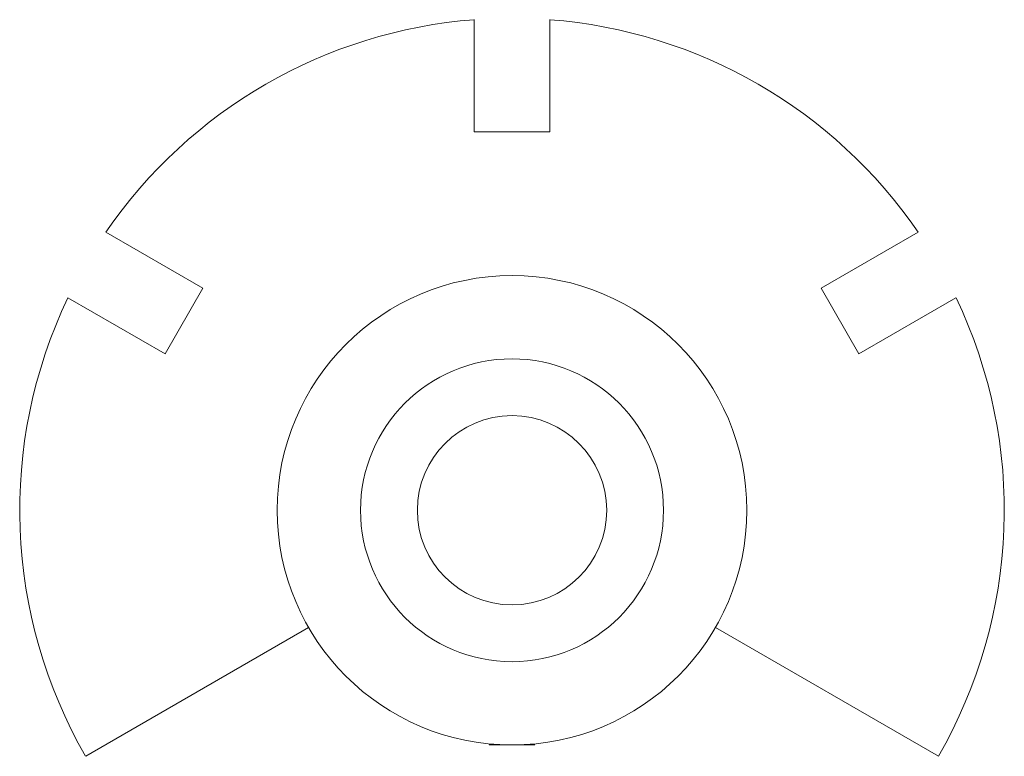
# Model space of a CAD drawing. Units: millimetres. Extents: x 3398 to 3528, y 1333 to 1430.
import ezdxf

# ---------------------------------------------------------------- set-up
doc = ezdxf.new("R2010")
doc.units = ezdxf.units.MM
doc.layers.add('M-CONS', color=8, linetype='Continuous', lineweight=18)

msp = doc.modelspace()

# ---------------------------------------------------------------- linework, layer by layer
at = {"layer": 'M-CONS'}
for p, q in [((3458.07, 1415.58), (3458.07, 1430.39)), ((3468.07, 1415.58), (3468.07, 1430.39)), ((3468.07, 1415.58), (3458.07, 1415.58)), ((3463.07, 1415.58), (3468.07, 1415.58)), ((3422.27, 1394.91), (3409.44, 1402.31)), ((3503.87, 1394.91), (3516.69, 1402.31)), ((3422.27, 1394.91), (3417.27, 1386.25)), ((3508.87, 1386.25), (3503.87, 1394.91)), ((3417.27, 1386.25), (3404.44, 1393.65)), ((3508.87, 1386.25), (3521.69, 1393.65)), ((3436.22, 1350.08), (3406.78, 1333.08)), ((3489.92, 1350.08), (3519.36, 1333.08))]:
    msp.add_line(p, q, dxfattribs=at)
for radius in [31, 20, 12.5]:
    msp.add_circle((3463.07, 1365.58), radius, dxfattribs=at)
at = {"layer": 'M-CONS', "extrusion": (0, -1, 0)}
msp.add_circle((3463.07, 30, -1334.58), 3, dxfattribs=at)
at = {"layer": 'M-CONS'}
for start, end in [(94.4117, 145.5883), (34.4117, 85.5883), (154.4117, 210), (330, 25.5883)]:
    msp.add_arc((3463.07, 1365.58), 65, start, end, dxfattribs=at)

doc.saveas('drawing.dxf')
